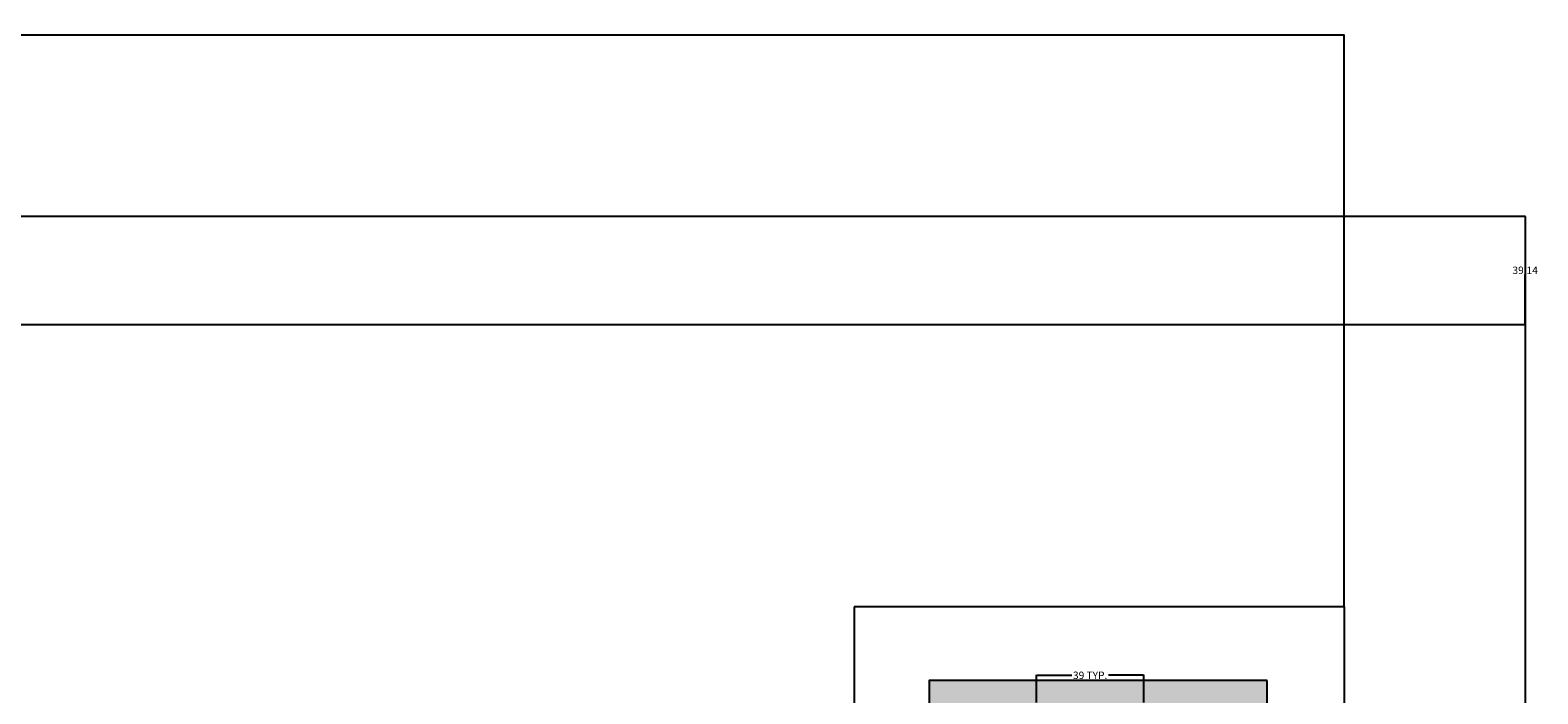
# Model space of a CAD drawing. Units: inches. Extents: x 2 to 1442, y 20 to 729.
# Tile 8 of 8: x 897 to 1441, y 489 to 729. Entities that reach past the tile are written whole.
import ezdxf

# ---------------------------------------------------------------- set-up
doc = ezdxf.new("R2010")
doc.units = ezdxf.units.IN
doc.header["$MEASUREMENT"] = 0
for name, color, linetype, lineweight in [('A-ANNO-DIMS', 2, 'Continuous', 18), ('A-ELEV', 7, 'Continuous', 25), ('A-WALL-PATT', 8, 'Continuous', 13)]:
    doc.layers.add(name, color=color, linetype=linetype, lineweight=lineweight)
doc.styles.get("Standard").update_dxf_attribs({"font": 'arial.ttf'})
doc.dimstyles.get("Standard").update_dxf_attribs({"dimtxt": 2.6875, "dimasz": 0.18, "dimexe": 0.18, "dimexo": 0.0625, "dimgap": 0.09, "dimtad": 0, "dimtih": 1, "dimtoh": 1, "dimdec": 4, "dimzin": 0, "dimdsep": 46, "dimlunit": 4, "dimtxsty": 'Standard', "dimcen": 0.09, "dimadec": 0, "dimazin": 0, "dimtfac": 1, "dimtdec": 4, "dimtofl": 0, "dimtmove": 0, "dimatfit": 3, "dimfxl": 1, "dimtolj": 1, "dimtzin": 0, "dimarcsym": 0})

# ---------------------------------------------------------------- blocks, each defined once
blk = doc.blocks.new('*D8')
at = {"layer": 'A-ANNO-DIMS', "color": 0, "lineweight": -2, "transparency": 16777216}
for p, q in [((1260.05, 486.08), (1260.05, 496.08)), ((1260.23, 495.9), (1272.79, 495.9)), ((1298.61, 495.9), (1286.05, 495.9)), ((1298.79, 486.08), (1298.79, 496.08))]:
    blk.add_line(p, q, dxfattribs=at)
at = {"layer": 'A-ANNO-DIMS', "color": 0, "transparency": 16777216}
for points in [[(1260.23, 495.93), (1260.23, 495.87), (1260.05, 495.9)], [(1298.61, 495.93), (1298.61, 495.87), (1298.79, 495.9)]]:
    blk.add_solid(points, dxfattribs=at)
at = {"layer": 'Defpoints', "color": 0, "transparency": 16777216}
for p in [(1298.79, 495.9), (1260.05, 486.02), (1298.79, 486.02)]:
    blk.add_point(p, dxfattribs=at)
at = {"layer": 'A-ANNO-DIMS', "color": 0, "transparency": 16777216, "insert": (1279.42, 495.9), "char_height": 2.6875, "attachment_point": 5}
blk.add_mtext('\\A1;39 TYP.', dxfattribs=at)
blk = doc.blocks.new('*D33')
at = {"layer": 'A-ANNO-DIMS', "color": 0, "lineweight": -2, "transparency": 16777216}
for p, q in [((722.06, 661.5), (1436.55, 661.5)), ((1436.37, 661.32), (1436.37, 375.85)), ((1436.37, 87.45), (1436.37, 372.92)), ((1371.19, 87.27), (1436.55, 87.27))]:
    blk.add_line(p, q, dxfattribs=at)
at = {"layer": 'A-ANNO-DIMS', "color": 0, "transparency": 16777216}
for points in [[(1436.34, 661.32), (1436.4, 661.32), (1436.37, 661.5)], [(1436.34, 87.45), (1436.4, 87.45), (1436.37, 87.27)]]:
    blk.add_solid(points, dxfattribs=at)
at = {"layer": 'Defpoints', "color": 0, "transparency": 16777216}
for p in [(722, 661.5), (1436.37, 661.5), (1371.12, 87.27)]:
    blk.add_point(p, dxfattribs=at)
at = {"layer": 'A-ANNO-DIMS', "color": 0, "transparency": 16777216, "insert": (1436.37, 374.39), "char_height": 2.688, "attachment_point": 5}
blk.add_mtext('\\A1;574.2', dxfattribs=at)
blk = doc.blocks.new('*D70')
at = {"layer": 'A-ANNO-DIMS', "color": 0, "lineweight": -2, "transparency": 16777216}
for p, q in [((722.06, 661.5), (1436.55, 661.5)), ((1436.37, 661.32), (1436.37, 643.39)), ((1436.37, 622.54), (1436.37, 640.47)), ((721.89, 622.36), (1436.55, 622.36))]:
    blk.add_line(p, q, dxfattribs=at)
at = {"layer": 'A-ANNO-DIMS', "color": 0, "transparency": 16777216}
for points in [[(1436.34, 661.32), (1436.4, 661.32), (1436.37, 661.5)], [(1436.34, 622.54), (1436.4, 622.54), (1436.37, 622.36)]]:
    blk.add_solid(points, dxfattribs=at)
at = {"layer": 'Defpoints', "color": 0, "transparency": 16777216}
for p in [(722, 661.5), (1436.37, 661.5), (721.83, 622.36)]:
    blk.add_point(p, dxfattribs=at)
at = {"layer": 'A-ANNO-DIMS', "color": 0, "transparency": 16777216, "insert": (1436.37, 641.93), "char_height": 2.688, "attachment_point": 5}
blk.add_mtext('\\A1;39.14', dxfattribs=at)
blk = doc.blocks.new('*D82')
at = {"layer": 'A-ANNO-DIMS', "color": 0, "lineweight": -2, "transparency": 16777216}
for p, q in [((72.53, 520.64), (72.53, 726.93)), ((72.71, 726.75), (716.28, 726.75)), ((1370.94, 726.75), (727.37, 726.75)), ((1371.12, 520.64), (1371.12, 726.93))]:
    blk.add_line(p, q, dxfattribs=at)
at = {"layer": 'A-ANNO-DIMS', "color": 0, "transparency": 16777216}
for points in [[(72.71, 726.78), (72.71, 726.72), (72.53, 726.75)], [(1370.94, 726.78), (1370.94, 726.72), (1371.12, 726.75)]]:
    blk.add_solid(points, dxfattribs=at)
at = {"layer": 'Defpoints', "color": 0, "transparency": 16777216}
for p in [(1371.12, 726.75), (72.53, 520.58), (1371.12, 520.58)]:
    blk.add_point(p, dxfattribs=at)
at = {"layer": 'A-ANNO-DIMS', "color": 0, "transparency": 16777216, "insert": (721.83, 726.75), "char_height": 2.688, "attachment_point": 5}
blk.add_mtext('\\A1;1298.6', dxfattribs=at)

msp = doc.modelspace()

# ---------------------------------------------------------------- hatches: boundary and pattern name
at = {"layer": 'A-WALL-PATT'}
h = msp.add_hatch(dxfattribs=at)
h.set_pattern_fill('BRASS', color=256, scale=14)
h.paths.add_polyline_path([(1221.296, 494.0357), (1343.2694, 494.0357), (1343.2694, 87.2714), (1325.228, 87.2714), (1325.228, 261.6116), (1313.3063, 261.6116), (1313.3063, 275.7919), (1313.3063, 320.992), (1313.3063, 322.0535), (1312.9828, 323.8227), (1310.4604, 330.4901), (1309.3395, 332.5101), (1304.6979, 338.5974), (1301.0035, 343.4423), (1299.8408, 344.5736), (1293.3137, 349.2734), (1292.0313, 349.9601), (1283.618, 353.1203), (1281.8598, 353.4396), (1279.7501, 353.4396), (1277.992, 353.1203), (1269.5786, 349.9601), (1268.2962, 349.2734), (1261.7691, 344.5736), (1260.6064, 343.4423), (1256.912, 338.5974), (1252.0504, 332.2216), (1251.278, 330.8295), (1248.6271, 323.8227), (1248.3037, 322.0535), (1248.3037, 320.992), (1248.3037, 276.0187), (1248.3037, 261.5562), (1236.3716, 261.5562), (1236.3716, 87.2714), (1221.296, 87.2714)])
h.paths.add_polyline_path([(1298.7943, 420.1495), (1298.7943, 464.3282), (1294.8674, 472.9254), (1285.9225, 481.8631), (1279.4227, 486.0178), (1272.9229, 481.8631), (1263.978, 472.9254), (1260.0512, 464.3282), (1260.0512, 420.1495)], flags=16)
h.paths.add_polyline_path([(1296.7943, 422.1495), (1296.7943, 463.893), (1293.1982, 471.7659), (1284.6625, 480.2948), (1279.4227, 483.6441), (1274.183, 480.2948), (1265.6472, 471.7659), (1262.0512, 463.893), (1262.0512, 422.1495)], flags=0)

# ---------------------------------------------------------------- linework, layer by layer
at = {"layer": 'A-ELEV'}
for p, q in [((1371.1242, 520.5823), (1194.3036, 520.5823)), ((1194.3036, 520.5823), (1194.3036, 471.2714)), ((1371.1242, 520.5823), (1371.1242, 464.6214))]:
    msp.add_line(p, q, dxfattribs=at)
msp.add_lwpolyline([(1343.2694, 494.0357), (1221.296, 494.0357), (1221.296, 87.2714), (1343.2694, 87.2714)], close=True, dxfattribs=at)

# ---------------------------------------------------------------- dimensions: what is measured, and where the dimension line sits
at = {"layer": 'A-ANNO-DIMS'}
dim = msp.add_linear_dim(base=(1371.1242, 726.75), p1=(72.5272, 520.5823), p2=(1371.1242, 520.5823), dimstyle='Standard', override={"dimdec": 1, "dimlfac": 1, "dimrnd": 0, "dimzin": 0, "dimdsep": 46, "dimlunit": 2}, dxfattribs=at)
dim.commit()
dim.dimension.update_dxf_attribs({"geometry": '*D82', "text_midpoint": (721.8257, 726.75)})
for p1, override, picture, middle in [((721.8257, 622.3576), {"dimdec": 2, "dimlfac": 1, "dimrnd": 0, "dimzin": 0, "dimdsep": 46, "dimlunit": 2}, '*D70', (1436.3742, 641.9288)), ((1371.1242, 87.2714), {"dimdec": 1, "dimlfac": 1, "dimrnd": 0, "dimzin": 0, "dimdsep": 46, "dimlunit": 2}, '*D33', (1436.3742, 374.3857))]:
    dim = msp.add_linear_dim(base=(1436.3742, 661.5), p1=p1, p2=(722, 661.5), angle=90, dimstyle='Standard', override=override, dxfattribs=at)
    dim.commit()
    dim.dimension.update_dxf_attribs({"geometry": picture, "text_midpoint": middle})
dim = msp.add_linear_dim(base=(1298.7943, 495.898), p1=(1260.0512, 486.0178), p2=(1298.7943, 486.0178), text='<> TYP.', dimstyle='Standard', override={"dimdec": 0, "dimrnd": 0, "dimzin": 0, "dimlunit": 2}, dxfattribs=at)
dim.commit()
dim.dimension.update_dxf_attribs({"geometry": '*D8', "text_midpoint": (1279.4227, 495.898)})

doc.saveas('drawing.dxf')
